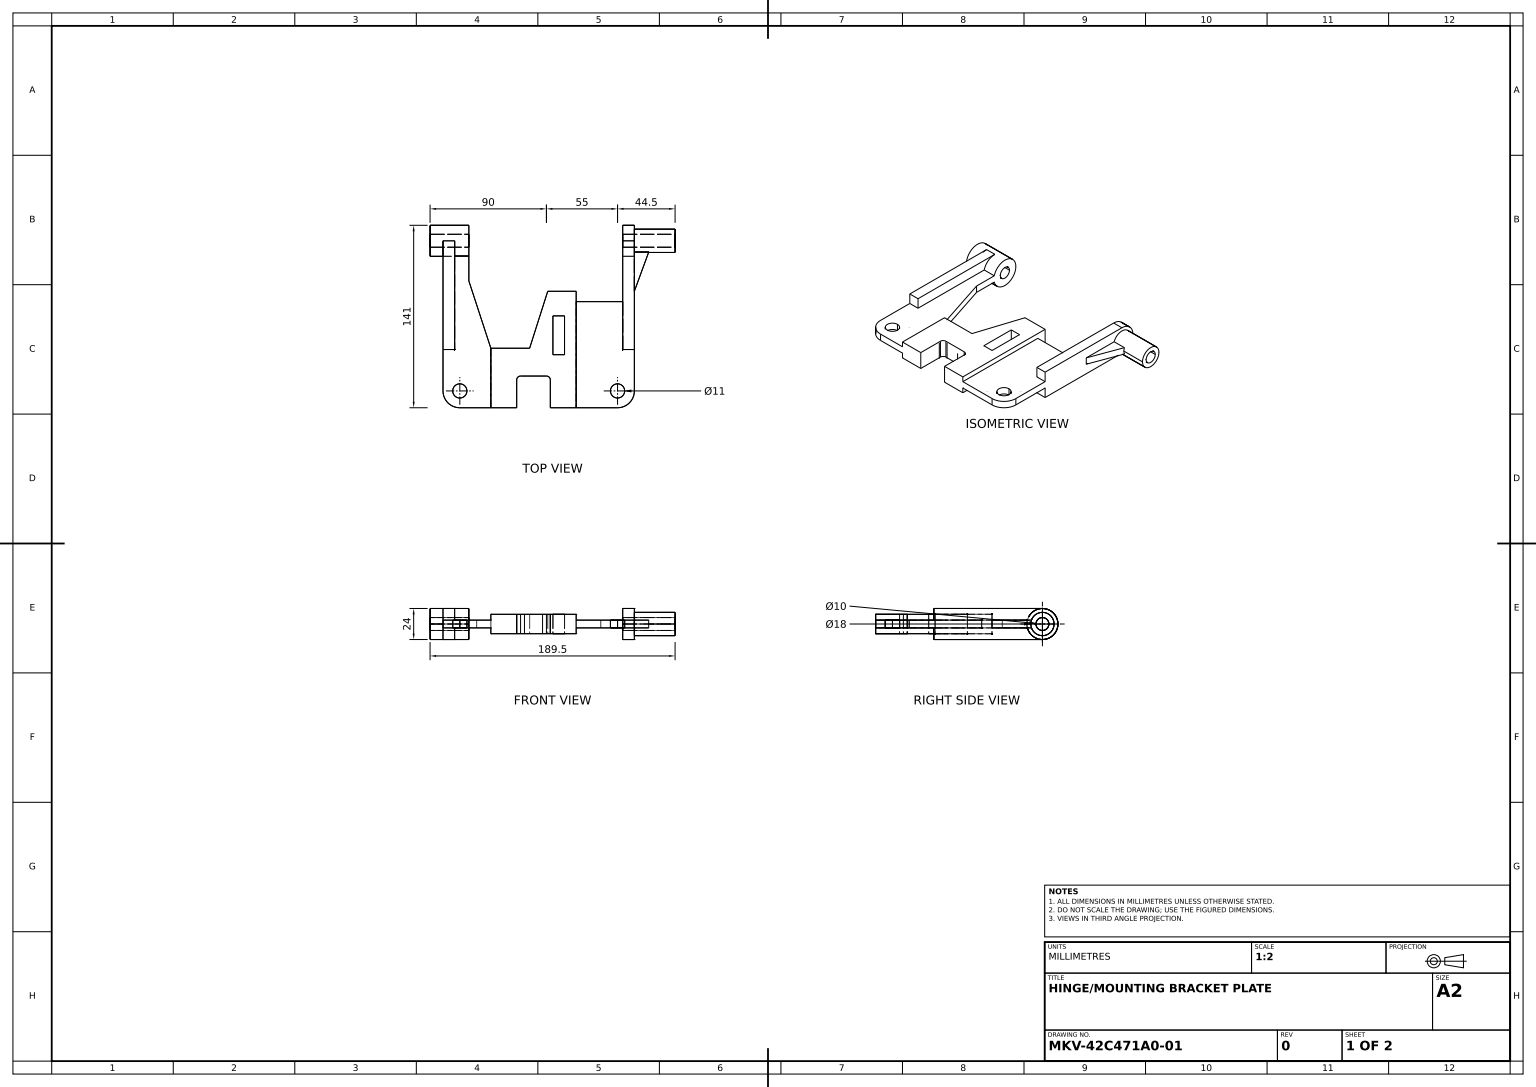
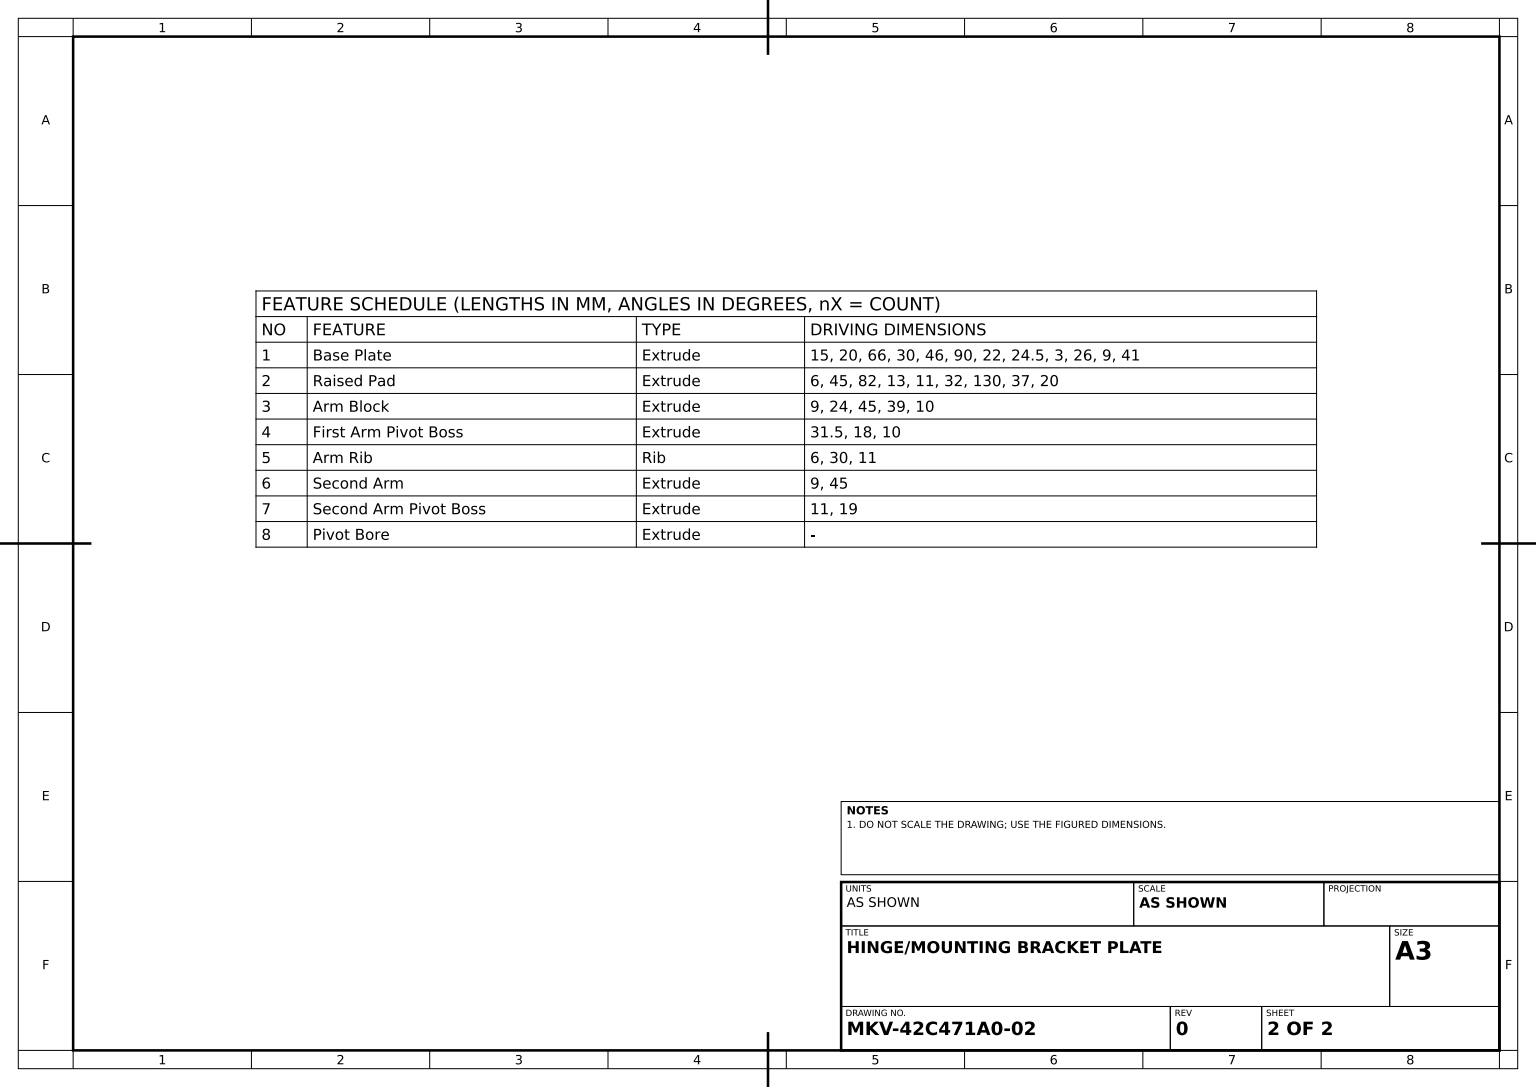
from build123d import *
from build123d.topology import SkipClean

# Parameters (mm, degrees)
BASE_PLATE_SKETCH_W              = 9
BASE_PLATE_SKETCH_H              = 30
BASE_PLATE_DEPTH                 = 7.5
RAISED_PAD_SKETCH_R              = 5.5
RAISED_PAD_DEPTH                 = 3
ARM_BLOCK_SKETCH_R               = 5
ARM_BLOCK_DEPTH                  = 9
FIRST_START                      = 31.5
FIRST_ARM_PIVOT_BOSS_SKETCH_R    = 9
FIRST_ARM_PIVOT_BOSS_SKETCH_R_2  = 5
FIRST_ARM_PIVOT_BOSS_DEPTH       = 31.5
ARM_RIB_REACH                    = 177.026
ARM_RIB_SKETCH_WALL_W            = 384.00451541
ARM_RIB_SKETCH_WALL_H            = 6
SECOND_START                     = -9
SECOND_ARM_DEPTH                 = 9
SECOND_ARM_PIVOT_BOSS_DEPTH      = 11
SECOND_ARM_PIVOT_BOSS_DEPTH_BACK = 19
SECOND_ARM_PIVOT_BOSS_SKETCH_R   = 12
PIVOT_BORE_SKETCH_R              = 5
PIVOT_BORE_DEPTH                 = 214.225819262


with BuildPart() as part:
    # Base Plate Sketch → Base Plate (new, symmetric)
    with BuildSketch(Plane(origin=(0, 0, 0), x_dir=(1, 0, 0), z_dir=(0, 1, 0))):
        with BuildLine():
            Line((-43, 24.5), (-23, 24.5))
            ThreePointArc((-23, 24.5), (-20.878679656, 23.621320344), (-20, 21.5))
            Line((-20, 21.5), (-20, 0))
            Line((-20, 0), (0, 0))
            Line((0, 0), (0, 90))
            Line((0, 90), (-22, 90))
            Line((-22, 90), (-36, 46))
            Line((-36, 46), (-66, 46))
            Line((-66, 46), (-66, 0))
            Line((-66, 0), (-46, 0))
            Line((-46, 0), (-46, 21.5))
            ThreePointArc((-46, 21.5), (-45.121320344, 23.621320344), (-43, 24.5))
        make_face()
        with Locations((-13.5, 56)):
            Rectangle(BASE_PLATE_SKETCH_W, BASE_PLATE_SKETCH_H, mode=Mode.SUBTRACT)
    extrude(amount=BASE_PLATE_DEPTH, both=True)

    # Raised Pad Sketch → Raised Pad (add, symmetric)
    # profile 1 of 2: a face of its own
    with BuildSketch(Plane(origin=(0, 0, 0), x_dir=(1, 0, 0), z_dir=(0, 1, 0))):
        with BuildLine():
            Line((0, 82), (45, 82))
            Line((45, 82), (45, 13))
            ThreePointArc((45, 13), (41.192388155, 3.807611845), (32, 0))
            Line((32, 0), (0, 0))
            Line((0, 0), (0, 82))
        make_face()
        with Locations(Location((32, 13, 0), (0, 0, 270))):
            Circle(RAISED_PAD_SKETCH_R, mode=Mode.SUBTRACT)
    # profile 2 of 2: a face of its own
    with BuildSketch(Plane(origin=(0, 0, 0), x_dir=(1, 0, 0), z_dir=(0, 1, 0))):
        with BuildLine():
            Line((-66, 0), (-90, 0))
            ThreePointArc((-90, 0), (-99.192388155, 3.807611845), (-103, 13))
            Line((-103, 13), (-103, 130))
            Line((-103, 130), (-83, 130))
            Line((-83, 130), (-83, 98))
            Line((-83, 98), (-66, 46))
            Line((-66, 46), (-66, 0))
        make_face()
        with Locations(Location((-90, 13, 0), (0, 0, 270))):
            Circle(RAISED_PAD_SKETCH_R, mode=Mode.SUBTRACT)
    extrude(amount=RAISED_PAD_DEPTH, both=True)

    # Arm Block Sketch → Arm Block (add)
    with BuildSketch(Plane(origin=(45, 0, 0), x_dir=(0, 0, -1), z_dir=(1, 0, 0))):
        with BuildLine():
            Line((45, 0), (45, 12))
            Line((45, 12), (129, 12))
            ThreePointArc((129, 12), (141, 0), (129, -12))
            Line((129, -12), (45, -12))
            Line((45, -12), (45, 0))
        make_face()
        with Locations((129, 0)):
            Circle(ARM_BLOCK_SKETCH_R, mode=Mode.SUBTRACT)
    extrude(amount=-ARM_BLOCK_DEPTH)

    # First Arm Pivot Boss Sketch → First Arm Pivot Boss (add)
    with BuildSketch(Plane(origin=(45, 0, 0), x_dir=(0, 0, -1), z_dir=(1, 0, 0)).offset(FIRST_START)):
        with Locations(Location((129, 0, 0), (0, 0, 180))):
            Circle(FIRST_ARM_PIVOT_BOSS_SKETCH_R)
        with Locations((129, 0)):
            Circle(FIRST_ARM_PIVOT_BOSS_SKETCH_R_2, mode=Mode.SUBTRACT)
    extrude(amount=-FIRST_ARM_PIVOT_BOSS_DEPTH)

    # Arm Rib Sketch wall → Arm Rib (add, up to next)
    with BuildSketch(Plane(origin=(50.5, 0, -105), x_dir=(0.344254649158, 0, -0.938876315887), z_dir=(-0.938876315887, 0, -0.344254649158)), mode=Mode.PRIVATE) as arm_rib_sk1:
        Rectangle(ARM_RIB_SKETCH_WALL_W, ARM_RIB_SKETCH_WALL_H)
    arm_rib_tool1 = extrude(arm_rib_sk1.sketch, amount=ARM_RIB_REACH, mode=Mode.PRIVATE) - part.part
    add(arm_rib_tool1.solids().sort_by_distance((50.5, 0, -105))[0])

    # Second Arm Sketch → Second Arm (add)
    with BuildSketch(Plane.ZY.offset(103).offset(SECOND_START)):
        with BuildLine():
            Line((-45, 0), (-45, 12))
            Line((-45, 12), (-129, 12))
            ThreePointArc((-129, 12), (-141, 0), (-129, -12))
            Line((-129, -12), (-45, -12))
            Line((-45, -12), (-45, 0))
        make_face()
    extrude(amount=SECOND_ARM_DEPTH)

    # Second Arm Pivot Boss Sketch → Second Arm Pivot Boss (add, two sides: drawn at the far end of the back side and taken through both)
    with SkipClean():  # the faces are left unmerged after this step: merging them gives an invalid solid
        with BuildSketch(Plane(origin=(-94, 0, 0), x_dir=(0, 0, -1), z_dir=(1, 0, 0)).offset(-SECOND_ARM_PIVOT_BOSS_DEPTH_BACK)):
            with Locations(Location((129, 0, 0), (0, 0, 194.477512186))):
                Circle(SECOND_ARM_PIVOT_BOSS_SKETCH_R)
        extrude(amount=SECOND_ARM_PIVOT_BOSS_DEPTH + SECOND_ARM_PIVOT_BOSS_DEPTH_BACK)

    # Pivot Bore Sketch → Pivot Bore (cut, through all)
    with SkipClean():  # the faces are left unmerged after this step: merging them gives an invalid solid
        with BuildSketch(Plane(origin=(-83, 0, 0), x_dir=(0, 0, -1), z_dir=(1, 0, 0))):
            with Locations((129, 0)):
                Circle(PIVOT_BORE_SKETCH_R)
        extrude(amount=-PIVOT_BORE_DEPTH, mode=Mode.SUBTRACT)


solid = part.part
